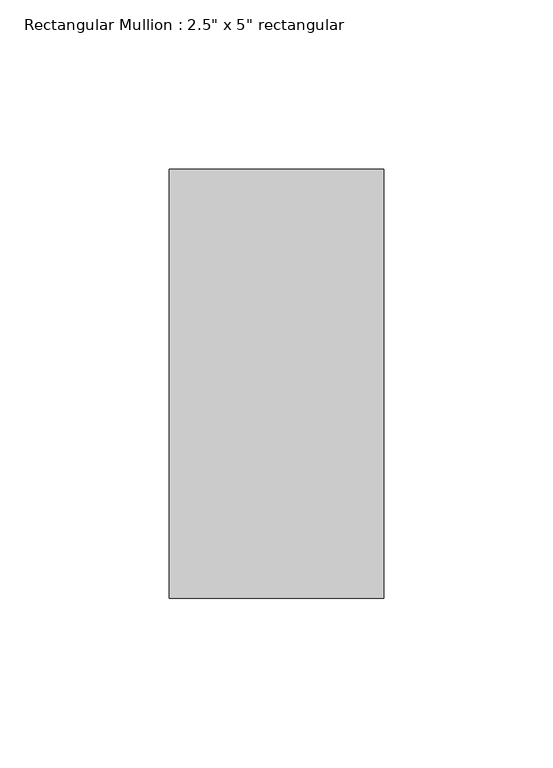
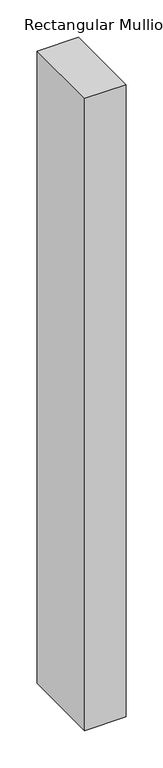
"""IFC4 building model written with IfcOpenShell, lengths in millimetres: member geometry."""

from ifc_helpers import new_model, si_unit, frame, origin, place, context, project, spatial, polyline, outline, extrude, source, transform, mapped, element, save


def member_02f15020(model_context):
    return source(origin(), model_context, "Body", "SweptSolid", [
        extrude(outline(polyline([(0.0, 63.5), (0.0, -63.5), (-63.5, -63.5), (-63.5, 63.5), (0.0, 63.5)])), frame((0.0, 0.0, -1031.7272807), z_axis=(0.0, 0.0, 1.0), x_axis=(1.0, 0.0, 0.0)), (0.0, 0.0, 1.0), 1031.7272807),
    ])


if __name__ == "__main__":
    model = new_model("IFC4")
    model_context = context("Model", 3, world=origin())
    ifc_project = project(units=[si_unit("LENGTHUNIT", "METRE", prefix="MILLI")], contexts=[model_context])
    site = spatial("IfcSite", under=ifc_project)
    building = spatial("IfcBuilding", under=site)
    placement = place(None, origin())
    member_shape = member_02f15020(model_context)
    element("IfcMember", 1, ObjectType="Rectangular Mullion : 2.5\" x 5\" rectangular", at=placement, inside=building, context=model_context, shape_type="MappedRepresentation", body=[
        mapped(member_shape, transform((0.0, 0.0, 0.0), x_axis=(1.0, 0.0, 0.0), y_axis=(0.0, 1.0, 0.0), z_axis=(0.0, 0.0, 1.0))),
    ])
    save(model, "model.ifc")

# Revit data of these elements
# Type "Rectangular Mullion : 2.5\" x 5\" rectangular"
#   built-in parameter 1007304 = 0.416667 (stored number, unit not read)
#   built-in parameter 1007301 = 0.104167 (stored number, unit not read)
#   built-in parameter 1007300 = 0.104167 (stored number, unit not read)
# Element 1 (IfcMember, "Rectangular Mullion : 2.5\" x 5\" rectangular")
#   Materials on its faces: "Aluminum"
# Materials
#   "Aluminum": class "Metal", colour RGB 247 247 247, transparency 0, Description = "Aluminum 6061", Cost = 0
